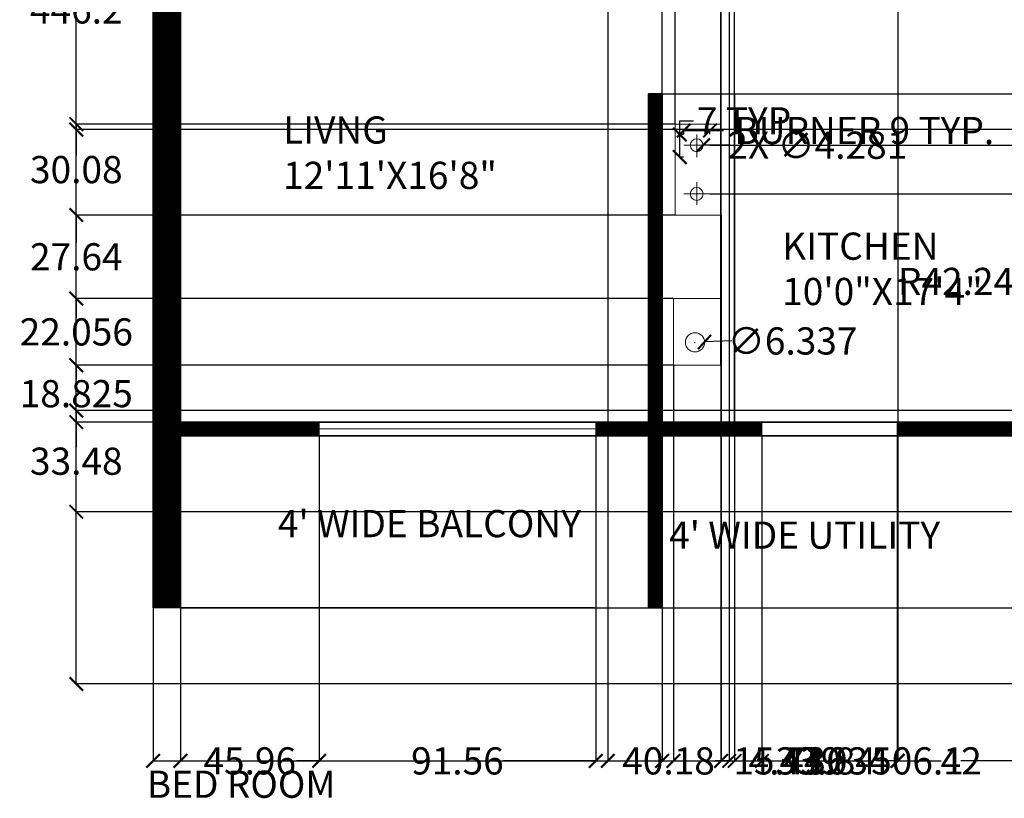
# Model space of a CAD drawing. Units: inches. Extents: x -43 to 552, y 22 to 537.
# Tile 1 of 4: x -43 to 283, y 22 to 280. Entities that reach past the tile are written whole.
import ezdxf

# ---------------------------------------------------------------- set-up
doc = ezdxf.new("R2010")
doc.units = ezdxf.units.IN
doc.header["$MEASUREMENT"] = 0
for name, color, linetype, lineweight in [('A-ANNO-DIMS', 2, 'Continuous', 18), ('A-AREA-IDEN', 7, 'Continuous', 18), ('A-EQPM', 8, 'Continuous', 18), ('A-FLOR', 7, 'Continuous', 25), ('A-FLOR-CASE', 8, 'Continuous', 25), ('A-FLOR-FIXT', 9, 'Continuous', 18), ('A-GLAZ', 4, 'Continuous', 18), ('A-WALL', 7, 'Continuous', 35), ('A-WALL-PATT', 252, 'Continuous', 13)]:
    doc.layers.add(name, color=color, linetype=linetype, lineweight=lineweight)
doc.styles.get("Standard").update_dxf_attribs({"font": 'arial.ttf'})
doc.dimstyles.get("Standard").update_dxf_attribs({"dimtxt": 9, "dimasz": 4.5, "dimexe": 0.18, "dimexo": 0.0625, "dimgap": 0.09, "dimtad": 0, "dimtih": 1, "dimtoh": 1, "dimdec": 1, "dimzin": 0, "dimdsep": 46, "dimlunit": 4, "dimtxsty": 'Standard', "dimblk": 'ARCHTICK', "dimcen": 0.09, "dimadec": 0, "dimazin": 0, "dimtfac": 1, "dimtdec": 1, "dimtofl": 0, "dimtmove": 0, "dimatfit": 3, "dimfxl": 1, "dimtolj": 1, "dimtzin": 0, "dimarcsym": 0})

# ---------------------------------------------------------------- blocks, each defined once
blk = doc.blocks.new('COOKTOP-BURNER')
for p, q in [((0, 0), (0, 3.57)), ((0, 3.57), (0, 0)), ((0, 0), (-4.28, 0)), ((0, 0), (4.4, 0)), ((0, 0), (0, -3.9))]:
    blk.add_line(p, q)
blk.add_circle((0, 0), 2.14)
blk = doc.blocks.new('_ArchTick')
at = {"color": 0, "linetype": 'ByBlock', "const_width": 0.15}
blk.add_lwpolyline([(-0.5, -0.5), (0.5, 0.5)], dxfattribs=at)
blk = doc.blocks.new('*D6')
at = {"layer": 'A-ANNO-DIMS', "color": 0, "lineweight": -2, "transparency": 16777216}
for p, q in [((177.13, 241.7), (177.13, 243.12)), ((177.13, 242.94), (185.81, 242.94)), ((185.81, 241.7), (185.81, 243.12)), ((185.81, 242.94), (190.31, 242.94))]:
    blk.add_line(p, q, dxfattribs=at)
at = {"layer": 'Defpoints', "color": 0, "transparency": 16777216}
for p in [(177.13, 241.64), (185.81, 242.94), (185.81, 241.64)]:
    blk.add_point(p, dxfattribs=at)
at = {"layer": 'A-ANNO-DIMS', "color": 0, "lineweight": -2, "transparency": 16777216, "xscale": 4.5, "yscale": 4.5, "zscale": 4.5, "rotation": 180}
blk.add_blockref('_ArchTick', (177.13, 242.94), dxfattribs=at)
at = {"layer": 'A-ANNO-DIMS', "color": 0, "lineweight": -2, "transparency": 16777216, "xscale": 4.5, "yscale": 4.5, "zscale": 4.5}
blk.add_blockref('_ArchTick', (185.81, 242.94), dxfattribs=at)
at = {"layer": 'A-ANNO-DIMS', "color": 0, "transparency": 16777216, "insert": (236.9, 242.94), "char_height": 9, "attachment_point": 5}
blk.add_mtext('\\A1;BURNER 9 TYP.', dxfattribs=at)
blk = doc.blocks.new('*D7')
at = {"layer": 'A-ANNO-DIMS', "color": 0, "lineweight": -2, "transparency": 16777216}
for p, q in [((175.83, 241.64), (175.83, 246.14)), ((175.83, 246.14), (180.33, 246.14)), ((177.07, 241.64), (175.65, 241.64)), ((175.83, 234.16), (175.83, 241.64)), ((177.07, 234.16), (175.65, 234.16))]:
    blk.add_line(p, q, dxfattribs=at)
at = {"layer": 'Defpoints', "color": 0, "transparency": 16777216}
for p in [(175.83, 241.64), (177.13, 241.64), (177.13, 234.16)]:
    blk.add_point(p, dxfattribs=at)
at = {"layer": 'A-ANNO-DIMS', "color": 0, "lineweight": -2, "transparency": 16777216, "xscale": 4.5, "yscale": 4.5, "zscale": 4.5}
for p, rotation in [((175.83, 241.64), 90), ((175.83, 234.16), 270)]:
    blk.add_blockref('_ArchTick', p, dxfattribs=dict(at, rotation=rotation))
at = {"layer": 'A-ANNO-DIMS', "color": 0, "transparency": 16777216, "insert": (198.79, 246.14), "char_height": 9, "attachment_point": 5}
blk.add_mtext('\\A1;7 TYP.', dxfattribs=at)
blk = doc.blocks.new('*D8')
at = {"layer": 'A-ANNO-DIMS', "color": 0, "lineweight": -2, "transparency": 16777216}
for p, q in [((507.56, 238.71), (507.56, 34.14)), ((1.46, 84.88), (1.46, 34.14)), ((1.46, 34.32), (240.11, 34.32)), ((507.56, 34.32), (268.92, 34.32))]:
    blk.add_line(p, q, dxfattribs=at)
at = {"layer": 'Defpoints', "color": 0, "transparency": 16777216}
for p in [(507.56, 238.77), (1.46, 84.95), (507.56, 34.32)]:
    blk.add_point(p, dxfattribs=at)
at = {"layer": 'A-ANNO-DIMS', "color": 0, "lineweight": -2, "transparency": 16777216, "xscale": 4.5, "yscale": 4.5, "zscale": 4.5, "rotation": 180}
blk.add_blockref('_ArchTick', (1.46, 34.32), dxfattribs=at)
at = {"layer": 'A-ANNO-DIMS', "color": 0, "lineweight": -2, "transparency": 16777216, "xscale": 4.5, "yscale": 4.5, "zscale": 4.5}
blk.add_blockref('_ArchTick', (507.56, 34.32), dxfattribs=at)
at = {"layer": 'A-ANNO-DIMS', "color": 0, "transparency": 16777216, "insert": (254.51, 34.32), "char_height": 9, "attachment_point": 5}
blk.add_mtext('\\A1;506.1', dxfattribs=at)
blk = doc.blocks.new('*D9')
at = {"layer": 'A-ANNO-DIMS', "color": 0, "lineweight": -2, "transparency": 16777216}
for p, q in [((82.45, 505.95), (-24.17, 505.95)), ((-23.99, 505.95), (-23.99, 287.55)), ((-23.99, 59.77), (-23.99, 278.18)), ((289.95, 59.77), (-24.17, 59.77))]:
    blk.add_line(p, q, dxfattribs=at)
at = {"layer": 'Defpoints', "color": 0, "transparency": 16777216}
for p in [(-23.99, 505.95), (82.51, 505.95), (290.01, 59.77)]:
    blk.add_point(p, dxfattribs=at)
at = {"layer": 'A-ANNO-DIMS', "color": 0, "lineweight": -2, "transparency": 16777216, "xscale": 4.5, "yscale": 4.5, "zscale": 4.5}
for p, rotation in [((-23.99, 505.95), 90), ((-23.99, 59.77), 270)]:
    blk.add_blockref('_ArchTick', p, dxfattribs=dict(at, rotation=rotation))
at = {"layer": 'A-ANNO-DIMS', "color": 0, "transparency": 16777216, "insert": (-23.99, 282.86), "char_height": 9, "attachment_point": 5}
blk.add_mtext('\\A1;446.2', dxfattribs=at)
blk = doc.blocks.new('*D22')
at = {"layer": 'A-ANNO-DIMS', "color": 0, "lineweight": -2, "transparency": 16777216}
for p, q in [((10.46, 141.88), (10.46, 34.14)), ((56.42, 141.88), (56.42, 34.14)), ((10.46, 34.32), (17.99, 34.32)), ((56.42, 34.32), (48.9, 34.32))]:
    blk.add_line(p, q, dxfattribs=at)
at = {"layer": 'Defpoints', "color": 0, "transparency": 16777216}
for p in [(10.46, 141.95), (56.42, 141.95), (56.42, 34.32)]:
    blk.add_point(p, dxfattribs=at)
at = {"layer": 'A-ANNO-DIMS', "color": 0, "lineweight": -2, "transparency": 16777216, "xscale": 4.5, "yscale": 4.5, "zscale": 4.5, "rotation": 180}
blk.add_blockref('_ArchTick', (10.46, 34.32), dxfattribs=at)
at = {"layer": 'A-ANNO-DIMS', "color": 0, "lineweight": -2, "transparency": 16777216, "xscale": 4.5, "yscale": 4.5, "zscale": 4.5}
blk.add_blockref('_ArchTick', (56.42, 34.32), dxfattribs=at)
at = {"layer": 'A-ANNO-DIMS', "color": 0, "transparency": 16777216, "insert": (33.44, 34.32), "char_height": 9, "attachment_point": 5}
blk.add_mtext('\\A1;45.96', dxfattribs=at)
blk = doc.blocks.new('*D23')
at = {"layer": 'A-ANNO-DIMS', "color": 0, "lineweight": -2, "transparency": 16777216}
for p, q in [((56.42, 141.88), (56.42, 34.14)), ((147.98, 141.88), (147.98, 34.14)), ((56.42, 34.32), (86.93, 34.32)), ((147.98, 34.32), (117.47, 34.32))]:
    blk.add_line(p, q, dxfattribs=at)
at = {"layer": 'Defpoints', "color": 0, "transparency": 16777216}
for p in [(56.42, 141.95), (147.98, 141.95), (147.98, 34.32)]:
    blk.add_point(p, dxfattribs=at)
at = {"layer": 'A-ANNO-DIMS', "color": 0, "lineweight": -2, "transparency": 16777216, "xscale": 4.5, "yscale": 4.5, "zscale": 4.5, "rotation": 180}
blk.add_blockref('_ArchTick', (56.42, 34.32), dxfattribs=at)
at = {"layer": 'A-ANNO-DIMS', "color": 0, "lineweight": -2, "transparency": 16777216, "xscale": 4.5, "yscale": 4.5, "zscale": 4.5}
blk.add_blockref('_ArchTick', (147.98, 34.32), dxfattribs=at)
at = {"layer": 'A-ANNO-DIMS', "color": 0, "transparency": 16777216, "insert": (102.2, 34.32), "char_height": 9, "attachment_point": 5}
blk.add_mtext('\\A1;91.56', dxfattribs=at)
blk = doc.blocks.new('*D26')
at = {"layer": 'A-ANNO-DIMS', "color": 0, "lineweight": -2, "transparency": 16777216}
for p, q in [((203, 141.88), (203, 34.14)), ((247.84, 141.88), (247.84, 34.14)), ((203, 34.32), (209.98, 34.32)), ((247.84, 34.32), (240.86, 34.32))]:
    blk.add_line(p, q, dxfattribs=at)
at = {"layer": 'Defpoints', "color": 0, "transparency": 16777216}
for p in [(203, 141.95), (247.84, 141.95), (247.84, 34.32)]:
    blk.add_point(p, dxfattribs=at)
at = {"layer": 'A-ANNO-DIMS', "color": 0, "lineweight": -2, "transparency": 16777216, "xscale": 4.5, "yscale": 4.5, "zscale": 4.5, "rotation": 180}
blk.add_blockref('_ArchTick', (203, 34.32), dxfattribs=at)
at = {"layer": 'A-ANNO-DIMS', "color": 0, "lineweight": -2, "transparency": 16777216, "xscale": 4.5, "yscale": 4.5, "zscale": 4.5}
blk.add_blockref('_ArchTick', (247.84, 34.32), dxfattribs=at)
at = {"layer": 'A-ANNO-DIMS', "color": 0, "transparency": 16777216, "insert": (225.42, 34.32), "char_height": 9, "attachment_point": 5}
blk.add_mtext('\\A1;44.84', dxfattribs=at)
blk = doc.blocks.new('*D27')
at = {"layer": 'A-ANNO-DIMS', "color": 0, "lineweight": -2, "transparency": 16777216}
for p, q in [((169.96, 141.88), (169.96, 34.14)), ((203, 141.88), (203, 34.14)), ((169.96, 34.32), (203, 34.32)), ((203, 34.32), (207.5, 34.32))]:
    blk.add_line(p, q, dxfattribs=at)
at = {"layer": 'Defpoints', "color": 0, "transparency": 16777216}
for p in [(169.96, 141.95), (203, 141.95), (203, 34.32)]:
    blk.add_point(p, dxfattribs=at)
at = {"layer": 'A-ANNO-DIMS', "color": 0, "lineweight": -2, "transparency": 16777216, "xscale": 4.5, "yscale": 4.5, "zscale": 4.5, "rotation": 180}
blk.add_blockref('_ArchTick', (169.96, 34.32), dxfattribs=at)
at = {"layer": 'A-ANNO-DIMS', "color": 0, "lineweight": -2, "transparency": 16777216, "xscale": 4.5, "yscale": 4.5, "zscale": 4.5}
blk.add_blockref('_ArchTick', (203, 34.32), dxfattribs=at)
at = {"layer": 'A-ANNO-DIMS', "color": 0, "transparency": 16777216, "insert": (226.25, 34.32), "char_height": 9, "attachment_point": 5}
blk.add_mtext('\\A1;33.034', dxfattribs=at)
blk = doc.blocks.new('*D29')
at = {"layer": 'A-ANNO-DIMS', "color": 0, "lineweight": -2, "transparency": 16777216}
for p, q in [((364.95, 346.45), (-24.17, 346.45)), ((-23.99, 346.45), (-23.99, 299.55)), ((-23.99, 243.27), (-23.99, 290.17)), ((364.95, 243.27), (-24.17, 243.27))]:
    blk.add_line(p, q, dxfattribs=at)
at = {"layer": 'Defpoints', "color": 0, "transparency": 16777216}
for p in [(-23.99, 346.45), (365.01, 346.45), (365.01, 243.27)]:
    blk.add_point(p, dxfattribs=at)
at = {"layer": 'A-ANNO-DIMS', "color": 0, "lineweight": -2, "transparency": 16777216, "xscale": 4.5, "yscale": 4.5, "zscale": 4.5}
for p, rotation in [((-23.99, 346.45), 90), ((-23.99, 243.27), 270)]:
    blk.add_blockref('_ArchTick', p, dxfattribs=dict(at, rotation=rotation))
at = {"layer": 'A-ANNO-DIMS', "color": 0, "transparency": 16777216, "insert": (-23.99, 294.86), "char_height": 9, "attachment_point": 5}
blk.add_mtext('\\A1;103.17', dxfattribs=at)
blk = doc.blocks.new('*D35')
at = {"layer": 'A-ANNO-DIMS', "color": 0, "lineweight": -2, "transparency": 16777216}
for p, q in [((10.53, 141.95), (533.19, 141.95)), ((533.01, 141.95), (533.01, 118.11)), ((533.01, 84.95), (533.01, 108.78)), ((10.53, 84.95), (533.19, 84.95))]:
    blk.add_line(p, q, dxfattribs=at)
at = {"layer": 'Defpoints', "color": 0, "transparency": 16777216}
for p in [(10.46, 141.95), (533.01, 141.95), (10.46, 84.95)]:
    blk.add_point(p, dxfattribs=at)
at = {"layer": 'A-ANNO-DIMS', "color": 0, "lineweight": -2, "transparency": 16777216, "xscale": 4.5, "yscale": 4.5, "zscale": 4.5}
for p, rotation in [((533.01, 141.95), 90), ((533.01, 84.95), 270)]:
    blk.add_blockref('_ArchTick', p, dxfattribs=dict(at, rotation=rotation))
at = {"layer": 'A-ANNO-DIMS', "color": 0, "transparency": 16777216, "insert": (533.01, 113.45), "char_height": 9, "attachment_point": 5}
blk.add_mtext('\\A1;57', dxfattribs=at)
blk = doc.blocks.new('*D37')
at = {"layer": 'A-ANNO-DIMS', "color": 0, "lineweight": -2, "transparency": 16777216}
for p, q in [((248.01, 346.38), (248.01, 34.14)), ((290.01, 346.38), (290.01, 34.14)), ((248.01, 34.32), (262.34, 34.32)), ((290.01, 34.32), (275.68, 34.32))]:
    blk.add_line(p, q, dxfattribs=at)
at = {"layer": 'Defpoints', "color": 0, "transparency": 16777216}
for p in [(248.01, 346.45), (290.01, 346.45), (290.01, 34.32)]:
    blk.add_point(p, dxfattribs=at)
at = {"layer": 'A-ANNO-DIMS', "color": 0, "lineweight": -2, "transparency": 16777216, "xscale": 4.5, "yscale": 4.5, "zscale": 4.5, "rotation": 180}
blk.add_blockref('_ArchTick', (248.01, 34.32), dxfattribs=at)
at = {"layer": 'A-ANNO-DIMS', "color": 0, "lineweight": -2, "transparency": 16777216, "xscale": 4.5, "yscale": 4.5, "zscale": 4.5}
blk.add_blockref('_ArchTick', (290.01, 34.32), dxfattribs=at)
at = {"layer": 'A-ANNO-DIMS', "color": 0, "transparency": 16777216, "insert": (269.01, 34.32), "char_height": 9, "attachment_point": 5}
blk.add_mtext('\\A1;42', dxfattribs=at)
blk = doc.blocks.new('*D39')
at = {"layer": 'A-ANNO-DIMS', "color": 0, "lineweight": -2, "transparency": 16777216}
for p, q in [((152.01, 496.88), (152.01, 34.14)), ((192.19, 486.68), (192.19, 34.14)), ((152.01, 34.32), (156.63, 34.32)), ((192.19, 34.32), (187.56, 34.32))]:
    blk.add_line(p, q, dxfattribs=at)
at = {"layer": 'Defpoints', "color": 0, "transparency": 16777216}
for p in [(152.01, 496.95), (192.19, 486.74), (192.19, 34.32)]:
    blk.add_point(p, dxfattribs=at)
at = {"layer": 'A-ANNO-DIMS', "color": 0, "lineweight": -2, "transparency": 16777216, "xscale": 4.5, "yscale": 4.5, "zscale": 4.5, "rotation": 180}
blk.add_blockref('_ArchTick', (152.01, 34.32), dxfattribs=at)
at = {"layer": 'A-ANNO-DIMS', "color": 0, "lineweight": -2, "transparency": 16777216, "xscale": 4.5, "yscale": 4.5, "zscale": 4.5}
blk.add_blockref('_ArchTick', (192.19, 34.32), dxfattribs=at)
at = {"layer": 'A-ANNO-DIMS', "color": 0, "transparency": 16777216, "insert": (172.1, 34.32), "char_height": 9, "attachment_point": 5}
blk.add_mtext('\\A1;40.18', dxfattribs=at)
blk = doc.blocks.new('*D43')
at = {"layer": 'A-ANNO-DIMS', "color": 0, "lineweight": -2, "transparency": 16777216}
for p, q in [((449.17, 150.25), (-24.17, 150.25)), ((-23.99, 150.25), (-23.99, 138.2)), ((-23.99, 116.77), (-23.99, 128.83)), ((468.45, 116.77), (-24.17, 116.77))]:
    blk.add_line(p, q, dxfattribs=at)
at = {"layer": 'Defpoints', "color": 0, "transparency": 16777216}
for p in [(-23.99, 150.25), (449.23, 150.25), (468.51, 116.77)]:
    blk.add_point(p, dxfattribs=at)
at = {"layer": 'A-ANNO-DIMS', "color": 0, "lineweight": -2, "transparency": 16777216, "xscale": 4.5, "yscale": 4.5, "zscale": 4.5}
for p, rotation in [((-23.99, 150.25), 90), ((-23.99, 116.77), 270)]:
    blk.add_blockref('_ArchTick', p, dxfattribs=dict(at, rotation=rotation))
at = {"layer": 'A-ANNO-DIMS', "color": 0, "transparency": 16777216, "insert": (-23.99, 133.51), "char_height": 9, "attachment_point": 5}
blk.add_mtext('\\A1;33.48', dxfattribs=at)
blk = doc.blocks.new('*D44')
at = {"layer": 'A-ANNO-DIMS', "color": 0, "lineweight": -2, "transparency": 16777216}
for p, q in [((169.96, 255.18), (169.96, 531.58)), ((169.96, 531.4), (175.37, 531.4)), ((193.96, 531.4), (188.56, 531.4)), ((193.96, 255.18), (193.96, 531.58))]:
    blk.add_line(p, q, dxfattribs=at)
at = {"layer": 'Defpoints', "color": 0, "transparency": 16777216}
for p in [(193.96, 531.4), (169.96, 255.12), (193.96, 255.12)]:
    blk.add_point(p, dxfattribs=at)
at = {"layer": 'A-ANNO-DIMS', "color": 0, "lineweight": -2, "transparency": 16777216, "xscale": 4.5, "yscale": 4.5, "zscale": 4.5, "rotation": 180}
blk.add_blockref('_ArchTick', (169.96, 531.4), dxfattribs=at)
at = {"layer": 'A-ANNO-DIMS', "color": 0, "lineweight": -2, "transparency": 16777216, "xscale": 4.5, "yscale": 4.5, "zscale": 4.5}
blk.add_blockref('_ArchTick', (193.96, 531.4), dxfattribs=at)
at = {"layer": 'A-ANNO-DIMS', "color": 0, "transparency": 16777216, "insert": (181.96, 531.4), "char_height": 9, "attachment_point": 5}
blk.add_mtext('\\A1;24', dxfattribs=at)
blk = doc.blocks.new('*D45')
at = {"layer": 'A-ANNO-DIMS', "color": 0, "lineweight": -2, "transparency": 16777216}
for p, q in [((194.03, 255.12), (533.19, 255.12)), ((533.01, 255.12), (533.01, 205.47)), ((533.01, 146.45), (533.01, 196.1)), ((194.03, 146.45), (533.19, 146.45))]:
    blk.add_line(p, q, dxfattribs=at)
at = {"layer": 'Defpoints', "color": 0, "transparency": 16777216}
for p in [(193.96, 255.12), (533.01, 255.12), (193.96, 146.45)]:
    blk.add_point(p, dxfattribs=at)
at = {"layer": 'A-ANNO-DIMS', "color": 0, "lineweight": -2, "transparency": 16777216, "xscale": 4.5, "yscale": 4.5, "zscale": 4.5}
for p, rotation in [((533.01, 255.12), 90), ((533.01, 146.45), 270)]:
    blk.add_blockref('_ArchTick', p, dxfattribs=dict(at, rotation=rotation))
at = {"layer": 'A-ANNO-DIMS', "color": 0, "transparency": 16777216, "insert": (533.01, 200.78), "char_height": 9, "attachment_point": 5}
blk.add_mtext('\\A1;108.67', dxfattribs=at)
blk = doc.blocks.new('*D46')
at = {"layer": 'A-ANNO-DIMS', "color": 0, "lineweight": -2, "transparency": 16777216}
for p, q in [((173.71, 165.21), (173.71, 34.14)), ((189.45, 165.21), (189.45, 34.14)), ((173.71, 34.32), (189.45, 34.32)), ((189.45, 34.32), (193.95, 34.32))]:
    blk.add_line(p, q, dxfattribs=at)
at = {"layer": 'Defpoints', "color": 0, "transparency": 16777216}
for p in [(173.71, 165.27), (189.45, 165.27), (189.45, 34.32)]:
    blk.add_point(p, dxfattribs=at)
at = {"layer": 'A-ANNO-DIMS', "color": 0, "lineweight": -2, "transparency": 16777216, "xscale": 4.5, "yscale": 4.5, "zscale": 4.5, "rotation": 180}
blk.add_blockref('_ArchTick', (173.71, 34.32), dxfattribs=at)
at = {"layer": 'A-ANNO-DIMS', "color": 0, "lineweight": -2, "transparency": 16777216, "xscale": 4.5, "yscale": 4.5, "zscale": 4.5}
blk.add_blockref('_ArchTick', (189.45, 34.32), dxfattribs=at)
at = {"layer": 'A-ANNO-DIMS', "color": 0, "transparency": 16777216, "insert": (212.29, 34.32), "char_height": 9, "attachment_point": 5}
blk.add_mtext('\\A1;15.736', dxfattribs=at)
blk = doc.blocks.new('*D47')
at = {"layer": 'A-ANNO-DIMS', "color": 0, "lineweight": -2, "transparency": 16777216}
for p, q in [((173.65, 187.33), (-24.17, 187.33)), ((-23.99, 187.33), (-23.99, 180.99)), ((-23.99, 165.27), (-23.99, 171.62)), ((173.65, 165.27), (-24.17, 165.27))]:
    blk.add_line(p, q, dxfattribs=at)
at = {"layer": 'Defpoints', "color": 0, "transparency": 16777216}
for p in [(-23.99, 187.33), (173.71, 187.33), (173.71, 165.27)]:
    blk.add_point(p, dxfattribs=at)
at = {"layer": 'A-ANNO-DIMS', "color": 0, "lineweight": -2, "transparency": 16777216, "xscale": 4.5, "yscale": 4.5, "zscale": 4.5}
for p, rotation in [((-23.99, 187.33), 90), ((-23.99, 165.27), 270)]:
    blk.add_blockref('_ArchTick', p, dxfattribs=dict(at, rotation=rotation))
at = {"layer": 'A-ANNO-DIMS', "color": 0, "transparency": 16777216, "insert": (-23.99, 176.3), "char_height": 9, "attachment_point": 5}
blk.add_mtext('\\A1;22.056', dxfattribs=at)
blk = doc.blocks.new('*D48')
at = {"layer": 'A-ANNO-DIMS', "color": 0, "lineweight": -2, "transparency": 16777216}
for p, q in [((174.25, 245.05), (-24.17, 245.05)), ((-23.99, 245.05), (-23.99, 234.7)), ((-23.99, 214.97), (-23.99, 225.32)), ((174.25, 214.97), (-24.17, 214.97))]:
    blk.add_line(p, q, dxfattribs=at)
at = {"layer": 'Defpoints', "color": 0, "transparency": 16777216}
for p in [(-23.99, 245.05), (174.31, 245.05), (174.31, 214.97)]:
    blk.add_point(p, dxfattribs=at)
at = {"layer": 'A-ANNO-DIMS', "color": 0, "lineweight": -2, "transparency": 16777216, "xscale": 4.5, "yscale": 4.5, "zscale": 4.5}
for p, rotation in [((-23.99, 245.05), 90), ((-23.99, 214.97), 270)]:
    blk.add_blockref('_ArchTick', p, dxfattribs=dict(at, rotation=rotation))
at = {"layer": 'A-ANNO-DIMS', "color": 0, "transparency": 16777216, "insert": (-23.99, 230.01), "char_height": 9, "attachment_point": 5}
blk.add_mtext('\\A1;30.08', dxfattribs=at)
blk = doc.blocks.new('*D49')
at = {"layer": 'A-ANNO-DIMS', "color": 0, "lineweight": -2, "transparency": 16777216}
for p, q in [((174.31, 245.11), (174.31, 531.58)), ((174.31, 531.4), (189.53, 531.4)), ((189.53, 245.11), (189.53, 531.58)), ((189.53, 531.4), (194.03, 531.4))]:
    blk.add_line(p, q, dxfattribs=at)
at = {"layer": 'Defpoints', "color": 0, "transparency": 16777216}
for p in [(189.53, 531.4), (174.31, 245.05), (189.53, 245.05)]:
    blk.add_point(p, dxfattribs=at)
at = {"layer": 'A-ANNO-DIMS', "color": 0, "lineweight": -2, "transparency": 16777216, "xscale": 4.5, "yscale": 4.5, "zscale": 4.5, "rotation": 180}
blk.add_blockref('_ArchTick', (174.31, 531.4), dxfattribs=at)
at = {"layer": 'A-ANNO-DIMS', "color": 0, "lineweight": -2, "transparency": 16777216, "xscale": 4.5, "yscale": 4.5, "zscale": 4.5}
blk.add_blockref('_ArchTick', (189.53, 531.4), dxfattribs=at)
at = {"layer": 'A-ANNO-DIMS', "color": 0, "transparency": 16777216, "insert": (212.37, 531.4), "char_height": 9, "attachment_point": 5}
blk.add_mtext('\\A1;15.216', dxfattribs=at)
blk = doc.blocks.new('*D50')
at = {"layer": 'A-ANNO-DIMS', "color": 0, "lineweight": -2, "transparency": 16777216}
for p, q in [((173.65, 165.27), (-24.17, 165.27)), ((-23.99, 165.27), (-23.99, 160.55)), ((-23.99, 146.45), (-23.99, 151.17)), ((169.9, 146.45), (-24.17, 146.45))]:
    blk.add_line(p, q, dxfattribs=at)
at = {"layer": 'Defpoints', "color": 0, "transparency": 16777216}
for p in [(-23.99, 165.27), (173.71, 165.27), (169.96, 146.45)]:
    blk.add_point(p, dxfattribs=at)
at = {"layer": 'A-ANNO-DIMS', "color": 0, "lineweight": -2, "transparency": 16777216, "xscale": 4.5, "yscale": 4.5, "zscale": 4.5}
for p, rotation in [((-23.99, 165.27), 90), ((-23.99, 146.45), 270)]:
    blk.add_blockref('_ArchTick', p, dxfattribs=dict(at, rotation=rotation))
at = {"layer": 'A-ANNO-DIMS', "color": 0, "transparency": 16777216, "insert": (-23.99, 155.86), "char_height": 9, "attachment_point": 5}
blk.add_mtext('\\A1;18.825', dxfattribs=at)
blk = doc.blocks.new('*D51')
at = {"layer": 'A-ANNO-DIMS', "color": 0, "lineweight": -2, "transparency": 16777216}
for p, q in [((174.25, 214.97), (-24.17, 214.97)), ((-23.99, 214.97), (-23.99, 205.83)), ((-23.99, 187.33), (-23.99, 196.46)), ((173.65, 187.33), (-24.17, 187.33))]:
    blk.add_line(p, q, dxfattribs=at)
at = {"layer": 'Defpoints', "color": 0, "transparency": 16777216}
for p in [(-23.99, 214.97), (174.31, 214.97), (173.71, 187.33)]:
    blk.add_point(p, dxfattribs=at)
at = {"layer": 'A-ANNO-DIMS', "color": 0, "lineweight": -2, "transparency": 16777216, "xscale": 4.5, "yscale": 4.5, "zscale": 4.5}
for p, rotation in [((-23.99, 214.97), 90), ((-23.99, 187.33), 270)]:
    blk.add_blockref('_ArchTick', p, dxfattribs=dict(at, rotation=rotation))
at = {"layer": 'A-ANNO-DIMS', "color": 0, "transparency": 16777216, "insert": (-23.99, 201.15), "char_height": 9, "attachment_point": 5}
blk.add_mtext('\\A1;27.64', dxfattribs=at)
blk = doc.blocks.new('*D52')
at = {"layer": 'A-ANNO-DIMS', "color": 0, "lineweight": -2, "transparency": 16777216}
for p, q in [((193.96, 255.05), (193.96, 34.14)), ((189.53, 214.91), (189.53, 34.14)), ((189.53, 34.32), (193.96, 34.32)), ((193.96, 34.32), (198.46, 34.32))]:
    blk.add_line(p, q, dxfattribs=at)
at = {"layer": 'Defpoints', "color": 0, "transparency": 16777216}
for p in [(193.96, 255.12), (189.53, 214.97), (193.96, 34.32)]:
    blk.add_point(p, dxfattribs=at)
at = {"layer": 'A-ANNO-DIMS', "color": 0, "lineweight": -2, "transparency": 16777216, "xscale": 4.5, "yscale": 4.5, "zscale": 4.5, "rotation": 180}
blk.add_blockref('_ArchTick', (189.53, 34.32), dxfattribs=at)
at = {"layer": 'A-ANNO-DIMS', "color": 0, "lineweight": -2, "transparency": 16777216, "xscale": 4.5, "yscale": 4.5, "zscale": 4.5}
blk.add_blockref('_ArchTick', (193.96, 34.32), dxfattribs=at)
at = {"layer": 'A-ANNO-DIMS', "color": 0, "transparency": 16777216, "insert": (213.93, 34.32), "char_height": 9, "attachment_point": 5}
blk.add_mtext('\\A1;4.439', dxfattribs=at)
blk = doc.blocks.new('*D53')
at = {"layer": 'A-ANNO-DIMS', "color": 0, "lineweight": -2, "transparency": 16777216}
for p, q in [((189.45, 165.34), (189.45, 531.58)), ((189.45, 531.4), (193.96, 531.4)), ((193.96, 146.51), (193.96, 531.58)), ((193.96, 531.4), (198.46, 531.4))]:
    blk.add_line(p, q, dxfattribs=at)
at = {"layer": 'Defpoints', "color": 0, "transparency": 16777216}
for p in [(193.96, 531.4), (189.45, 165.27), (193.96, 146.45)]:
    blk.add_point(p, dxfattribs=at)
at = {"layer": 'A-ANNO-DIMS', "color": 0, "lineweight": -2, "transparency": 16777216, "xscale": 4.5, "yscale": 4.5, "zscale": 4.5, "rotation": 180}
blk.add_blockref('_ArchTick', (189.45, 531.4), dxfattribs=at)
at = {"layer": 'A-ANNO-DIMS', "color": 0, "lineweight": -2, "transparency": 16777216, "xscale": 4.5, "yscale": 4.5, "zscale": 4.5}
blk.add_blockref('_ArchTick', (193.96, 531.4), dxfattribs=at)
at = {"layer": 'A-ANNO-DIMS', "color": 0, "transparency": 16777216, "insert": (210.38, 531.4), "char_height": 9, "attachment_point": 5}
blk.add_mtext('\\A1;4.52', dxfattribs=at)
blk = doc.blocks.new('*D54')
at = {"layer": 'A-ANNO-DIMS', "color": 0, "lineweight": -2, "transparency": 16777216}
for p, q in [((185.87, 238.07), (533.19, 238.07)), ((533.01, 238.07), (533.01, 234.7)), ((533.01, 221.96), (533.01, 225.33)), ((185.87, 221.96), (533.19, 221.96))]:
    blk.add_line(p, q, dxfattribs=at)
at = {"layer": 'Defpoints', "color": 0, "transparency": 16777216}
for p in [(185.81, 238.07), (533.01, 238.07), (185.81, 221.96)]:
    blk.add_point(p, dxfattribs=at)
at = {"layer": 'A-ANNO-DIMS', "color": 0, "lineweight": -2, "transparency": 16777216, "xscale": 4.5, "yscale": 4.5, "zscale": 4.5}
for p, rotation in [((533.01, 238.07), 90), ((533.01, 221.96), 270)]:
    blk.add_blockref('_ArchTick', p, dxfattribs=dict(at, rotation=rotation))
at = {"layer": 'A-ANNO-DIMS', "color": 0, "transparency": 16777216, "insert": (533.01, 230.01), "char_height": 9, "attachment_point": 5}
blk.add_mtext('\\A1;16.11', dxfattribs=at)
blk = doc.blocks.new('*D57')
at = {"layer": 'A-ANNO-DIMS', "color": 0, "lineweight": -2, "transparency": 16777216}
for p, q in [((336.42, 243.27), (336.6, 243.27)), ((336.51, 243.18), (336.51, 243.36)), ((291.34, 193), (308.28, 211.86)), ((286.84, 193), (291.34, 193))]:
    blk.add_line(p, q, dxfattribs=at)
at = {"layer": 'Defpoints', "color": 0, "transparency": 16777216}
for p in [(336.51, 243.27), (308.28, 211.86)]:
    blk.add_point(p, dxfattribs=at)
at = {"layer": 'A-ANNO-DIMS', "color": 0, "lineweight": -2, "transparency": 16777216, "xscale": 4.5, "yscale": 4.5, "zscale": 4.5, "rotation": 48.05760462108148}
blk.add_blockref('_ArchTick', (308.28, 211.86), dxfattribs=at)
at = {"layer": 'A-ANNO-DIMS', "color": 0, "transparency": 16777216, "insert": (267.27, 193), "char_height": 9, "attachment_point": 5}
blk.add_mtext('\\A1;R42.24', dxfattribs=at)
blk = doc.blocks.new('*D59')
at = {"layer": 'A-ANNO-DIMS', "color": 0, "lineweight": -2, "transparency": 16777216}
for p, q in [((180.75, 172.84), (180.93, 172.84)), ((180.84, 172.75), (180.84, 172.93)), ((193, 173.3), (184.01, 172.96))]:
    blk.add_line(p, q, dxfattribs=at)
at = {"layer": 'Defpoints', "color": 0, "transparency": 16777216}
for p in [(184.01, 172.96), (177.68, 172.72)]:
    blk.add_point(p, dxfattribs=at)
at = {"layer": 'A-ANNO-DIMS', "color": 0, "lineweight": -2, "transparency": 16777216, "xscale": 4.5, "yscale": 4.5, "zscale": 4.5, "rotation": 182.1701531593034}
blk.add_blockref('_ArchTick', (184.01, 172.96), dxfattribs=at)
at = {"layer": 'A-ANNO-DIMS', "color": 0, "transparency": 16777216, "insert": (213.18, 173.3), "char_height": 9, "attachment_point": 5}
blk.add_mtext('\\A1;∅6.337', dxfattribs=at)
blk = doc.blocks.new('*D60')
at = {"layer": 'A-ANNO-DIMS', "color": 0, "lineweight": -2, "transparency": 16777216}
for p, q in [((181.32, 238.07), (181.5, 238.07)), ((181.41, 237.98), (181.41, 238.16)), ((192.55, 238.09), (183.55, 238.07))]:
    blk.add_line(p, q, dxfattribs=at)
at = {"layer": 'Defpoints', "color": 0, "transparency": 16777216}
for p in [(179.27, 238.06), (183.55, 238.07)]:
    blk.add_point(p, dxfattribs=at)
at = {"layer": 'A-ANNO-DIMS', "color": 0, "lineweight": -2, "transparency": 16777216, "xscale": 4.5, "yscale": 4.5, "zscale": 4.5, "rotation": 180.1229965869815}
blk.add_blockref('_ArchTick', (183.55, 238.07), dxfattribs=at)
at = {"layer": 'A-ANNO-DIMS', "color": 0, "transparency": 16777216, "insert": (221.36, 238.09), "char_height": 9, "attachment_point": 5}
blk.add_mtext('\\A1;2X ∅4.281', dxfattribs=at)

msp = doc.modelspace()

# ---------------------------------------------------------------- hatches: boundary and pattern name
at = {"layer": 'A-WALL-PATT'}
h = msp.add_hatch(dxfattribs=at)
h.set_pattern_fill('ANSI31', color=256)
h.set_pattern_definition([(45, (-523.11303, 0), (-0.088388348, 0.088388348), [])])
h.paths.add_polyline_path([(202.9985, 146.4471), (169.965, 146.4471), (169.965, 255.1157), (165.465, 255.1157), (165.465, 146.4471), (147.9805, 146.4471), (147.9805, 141.9471), (165.465, 141.9471), (165.465, 84.9471), (169.965, 84.9471), (169.965, 141.9471), (202.9985, 141.9471)])
h.paths.add_polyline_path([(294.5106, 146.4471), (294.5106, 238.775), (294.5106, 243.275), (294.5106, 255.1157), (290.0106, 255.1157), (290.0106, 146.4471), (247.8411, 146.4471), (247.8411, 141.9471), (290.0106, 141.9471), (290.0106, 93.9471), (290.0106, 59.775), (294.5106, 59.775), (294.5106, 77.3814), (294.5106, 93.9471), (294.5106, 107.775), (316.2676, 107.775), (316.2676, 116.775), (294.5106, 116.775)])
h.paths.add_polyline_path([(10.465, 346.4471), (82.5106, 346.4471), (91.5106, 346.4471), (91.5106, 358.2163), (82.5106, 358.2163), (82.5106, 350.9471), (1.465, 350.9471), (1.465, 84.9471), (10.465, 84.9471), (10.465, 141.9471), (56.4237, 141.9471), (56.4237, 146.4471), (10.465, 146.4471)])
h.paths.add_polyline_path([(91.5106, 496.9471), (107.5106, 496.9471), (107.5106, 505.9471), (82.5106, 505.9471), (82.5106, 400.4471), (147.5106, 400.4471), (147.5106, 346.4471), (248.0106, 346.4471), (248.0106, 350.9471), (152.0106, 350.9471), (152.0106, 496.9471), (197.0106, 496.9471), (197.0106, 505.9471), (131.5106, 505.9471), (131.5106, 496.9471), (147.5106, 496.9471), (147.5106, 404.9471), (91.5106, 404.9471)])
h.paths.add_polyline_path([(477.5106, 505.9471), (245.0106, 505.9471), (245.0106, 496.9471), (290.0106, 496.9471), (290.0106, 390.2693, -0.02565505), (294.5106, 390.2693), (294.5106, 496.9471), (468.5106, 496.9471), (468.5106, 460.1763), (477.5106, 460.1763)])

# ---------------------------------------------------------------- linework, layer by layer
at = {"layer": 'A-EQPM'}
for p, q in [((174.3101, 245.0503), (189.5259, 245.0503)), ((174.3101, 214.9706), (174.3101, 245.0503)), ((189.5259, 245.0503), (189.5259, 214.9706)), ((189.5259, 214.9706), (174.3101, 214.9706))]:
    msp.add_line(p, q, dxfattribs=at)
at = {"layer": 'A-FLOR'}
for q in [(1.465, 84.9471), (290.0106, 84.9471)]:
    msp.add_line((147.5106, 84.9471), q, dxfattribs=at)
at = {"layer": 'A-FLOR-CASE'}
for p, q in [((169.965, 255.1157), (193.965, 255.1157)), ((193.965, 255.1157), (193.965, 146.4471))]:
    msp.add_line(p, q, dxfattribs=at)
at = {"layer": 'A-FLOR-FIXT'}
msp.add_lwpolyline([(173.7137, 187.3286), (189.4495, 187.3286), (189.4495, 165.2726), (173.7137, 165.2726)], close=True, dxfattribs=at)
msp.add_circle((180.8445, 172.838), 3.1685, dxfattribs=at)
at = {"layer": 'A-GLAZ'}
for p, q in [((56.4237, 146.4471), (56.4237, 141.9471)), ((56.4237, 144.1971), (147.9805, 144.1971)), ((147.9805, 146.4471), (147.9805, 141.9471)), ((202.9985, 146.4471), (202.9985, 141.9471)), ((247.8411, 146.4471), (247.8411, 141.9471))]:
    msp.add_line(p, q, dxfattribs=at)
at = {"layer": 'A-WALL'}
for p, q in [((1.465, 350.9471), (1.465, 84.9471)), ((10.465, 346.4471), (10.465, 146.4471)), ((165.465, 255.1157), (165.465, 146.4471)), ((169.965, 255.1157), (165.465, 255.1157)), ((169.965, 255.1157), (169.965, 146.4471)), ((82.5106, 146.4471), (10.465, 146.4471)), ((82.5106, 146.4471), (165.465, 146.4471)), ((169.965, 146.4471), (290.0106, 146.4471)), ((82.5106, 141.9471), (10.465, 141.9471)), ((10.465, 141.9471), (10.465, 84.9471)), ((82.5106, 141.9471), (165.465, 141.9471)), ((165.465, 141.9471), (165.465, 84.9471)), ((169.965, 141.9471), (169.965, 84.9471)), ((169.965, 141.9471), (290.0106, 141.9471))]:
    msp.add_line(p, q, dxfattribs=at)

# ---------------------------------------------------------------- block references
at = {"layer": 'A-EQPM'}
msp.add_blockref('COOKTOP-BURNER', (181.4108, 238.0655), dxfattribs=at)
at = {"layer": 'A-EQPM', "extrusion": (0, 0, -1), "zscale": -1, "rotation": 180}
msp.add_blockref('COOKTOP-BURNER', (-181.4108, 221.9554), dxfattribs=at)

# ---------------------------------------------------------------- texts
at = {"layer": 'A-AREA-IDEN', "char_height": 9, "attachment_point": 1}
for s, insert in [('LIVNG\\P12\'11\'X16\'8"', (44.48, 247.6139)), ('KITCHEN\\P10\'0"X17\'4"', (209.721, 209.1705)), ("4' WIDE BALCONY", (42.7425, 117.3453)), ("4' WIDE UTILITY", (172.2793, 113.5372)), ('BED ROOM', (-0.6528, 31.0994))]:
    msp.add_mtext_dynamic_manual_height_columns(s, width=549.697564, gutter_width=1, heights=[0], dxfattribs=dict(at, insert=insert))

# ---------------------------------------------------------------- dimensions: what is measured, and where the dimension line sits
at = {"layer": 'A-ANNO-DIMS'}
for base, p1, p2, override, picture, middle in [((193.965, 531.3971), (169.965, 255.1157), (193.965, 255.1157), {"dimdec": 0, "dimlfac": 1, "dimrnd": 0, "dimzin": 0, "dimdsep": 46, "dimlunit": 2}, '*D44', (181.965, 531.3971)), ((189.5259, 531.3971), (174.3101, 245.0503), (189.5259, 245.0503), {"dimdec": 3, "dimlfac": 1, "dimrnd": 0, "dimzin": 0, "dimdsep": 46, "dimlunit": 2}, '*D49', (212.3707, 531.3971)), ((193.965, 531.3971), (189.4495, 165.2726), (193.965, 146.4471), {"dimdec": 2, "dimlfac": 1, "dimrnd": 0, "dimzin": 0, "dimdsep": 46, "dimlunit": 2}, '*D53', (210.379, 531.3971)), ((192.1876, 34.325), (152.0106, 496.9471), (192.1876, 486.7427), {"dimdec": 2, "dimlfac": 1, "dimrnd": 0, "dimzin": 0, "dimdsep": 46, "dimlunit": 2}, '*D39', (172.0991, 34.325)), ((290.0106, 34.325), (248.0106, 346.4471), (290.0106, 346.4471), {"dimdec": 0, "dimlfac": 1, "dimrnd": 0, "dimzin": 0, "dimdsep": 46, "dimlunit": 2}, '*D37', (269.0106, 34.325)), ((193.965, 34.325), (189.5259, 214.9706), (193.965, 255.1157), {"dimdec": 3, "dimlfac": 1, "dimrnd": 0, "dimzin": 0, "dimdsep": 46, "dimlunit": 2}, '*D52', (213.9305, 34.325)), ((507.5611, 34.325), (1.465, 84.9471), (507.5611, 238.775), {"dimdec": 1, "dimlfac": 1, "dimrnd": 0, "dimzin": 0, "dimdsep": 46, "dimlunit": 2}, '*D8', (254.513, 34.325)), ((189.4495, 34.325), (173.7137, 165.2726), (189.4495, 165.2726), {"dimdec": 3, "dimlfac": 1, "dimrnd": 0, "dimzin": 0, "dimdsep": 46, "dimlunit": 2}, '*D46', (212.2942, 34.325)), ((56.4237, 34.325), (10.465, 141.9471), (56.4237, 141.9471), {"dimdec": 2, "dimlfac": 1, "dimrnd": 0, "dimzin": 0, "dimdsep": 46, "dimlunit": 2}, '*D22', (33.4443, 34.325)), ((147.9805, 34.325), (56.4237, 141.9471), (147.9805, 141.9471), {"dimdec": 2, "dimlfac": 1, "dimrnd": 0, "dimzin": 0, "dimdsep": 46, "dimlunit": 2}, '*D23', (102.2021, 34.325)), ((202.99846, 34.32496), (169.96495, 141.94715), (202.99846, 141.94715), {"dimdec": 3, "dimlfac": 1, "dimrnd": 0, "dimzin": 0, "dimdsep": 46, "dimlunit": 2}, '*D27', (226.24842, 34.32496)), ((247.8411, 34.325), (202.9985, 141.9471), (247.8411, 141.9471), {"dimdec": 2, "dimlfac": 1, "dimrnd": 0, "dimzin": 0, "dimdsep": 46, "dimlunit": 2}, '*D26', (225.4198, 34.325))]:
    dim = msp.add_linear_dim(base=base, p1=p1, p2=p2, dimstyle='Standard', override=override, dxfattribs=at)
    dim.commit()
    dim.dimension.update_dxf_attribs({"geometry": picture, "text_midpoint": middle})
for base, p1, p2, override, picture, middle in [((-23.985, 505.9471), (290.0106, 59.775), (82.5106, 505.9471), {"dimdec": 1, "dimlfac": 1, "dimrnd": 0, "dimzin": 0, "dimdsep": 46, "dimlunit": 2}, '*D9', (-23.985, 282.8611)), ((-23.985, 346.4471), (365.0106, 243.275), (365.0106, 346.4471), {"dimdec": 2, "dimlfac": 1, "dimrnd": 0, "dimzin": 0, "dimdsep": 46, "dimlunit": 2}, '*D29', (-23.985, 294.8611)), ((533.0111, 255.1157), (193.965, 146.4471), (193.965, 255.1157), {"dimdec": 2, "dimlfac": 1, "dimrnd": 0, "dimzin": 0, "dimdsep": 46, "dimlunit": 2}, '*D45', (533.0111, 200.7814)), ((-23.985, 245.0503), (174.3101, 214.9706), (174.3101, 245.0503), {"dimdec": 2, "dimlfac": 1, "dimrnd": 0, "dimzin": 0, "dimdsep": 46, "dimlunit": 2}, '*D48', (-23.985, 230.0105)), ((533.0111, 238.0655), (185.8076, 221.9554), (185.8076, 238.0655), {"dimdec": 2, "dimlfac": 1, "dimrnd": 0, "dimzin": 0, "dimdsep": 46, "dimlunit": 2}, '*D54', (533.0111, 230.0105)), ((-23.985, 214.9706), (173.7137, 187.3286), (174.3101, 214.9706), {"dimdec": 2, "dimlfac": 1, "dimrnd": 0, "dimzin": 0, "dimdsep": 46, "dimlunit": 2}, '*D51', (-23.985, 201.1496)), ((-23.985, 187.3286), (173.7137, 165.2726), (173.7137, 187.3286), {"dimdec": 3, "dimlfac": 1, "dimrnd": 0, "dimzin": 0, "dimdsep": 46, "dimlunit": 2}, '*D47', (-23.985, 176.3006)), ((-23.98505, 165.27256), (169.96495, 146.44715), (173.71369, 165.27256), {"dimdec": 3, "dimlfac": 1, "dimrnd": 0, "dimzin": 0, "dimdsep": 46, "dimlunit": 2}, '*D50', (-23.98505, 155.85985)), ((-23.985, 150.2529), (468.5106, 116.775), (449.2346, 150.2529), {"dimdec": 2, "dimlfac": 1, "dimrnd": 0, "dimzin": 0, "dimdsep": 46, "dimlunit": 2}, '*D43', (-23.985, 133.5139)), ((533.0111, 141.9471), (10.465, 84.9471), (10.465, 141.9471), {"dimdec": 0, "dimlfac": 1, "dimrnd": 0, "dimzin": 0, "dimdsep": 46, "dimlunit": 2}, '*D35', (533.0111, 113.4471))]:
    dim = msp.add_linear_dim(base=base, p1=p1, p2=p2, angle=90, dimstyle='Standard', override=override, dxfattribs=at)
    dim.commit()
    dim.dimension.update_dxf_attribs({"geometry": picture, "text_midpoint": middle})
dim = msp.add_linear_dim(base=(185.8076, 242.9397), p1=(177.1301, 241.6381), p2=(185.8076, 241.6381), text='BURNER <> TYP.', dimstyle='Standard', override={"dimdec": 0, "dimlfac": 1, "dimrnd": 0, "dimzin": 0, "dimdsep": 46, "dimlunit": 2}, dxfattribs=at)
dim.commit()
dim.dimension.update_dxf_attribs({"geometry": '*D6', "text_midpoint": (236.8986, 242.9397)})
dim = msp.add_linear_dim(base=(175.8285, 241.6381), p1=(177.1301, 234.1635), p2=(177.1301, 241.6381), angle=90, text='<> TYP.', dimstyle='Standard', override={"dimdec": 0, "dimlfac": 1, "dimrnd": 0, "dimzin": 0, "dimdsep": 46, "dimlunit": 2}, dxfattribs=at)
dim.commit()
dim.dimension.update_dxf_attribs({"geometry": '*D7', "text_midpoint": (198.7899, 246.1381)})
dim = msp.add_diameter_dim_2p(p1=(179.2703, 238.0609), p2=(183.5513, 238.0701), text='2X <>', dimstyle='Standard', override={"dimdec": 3, "dimlfac": 1, "dimrnd": 0, "dimzin": 0, "dimdsep": 46, "dimlunit": 2}, dxfattribs=at)
dim.commit()
dim.dimension.update_dxf_attribs({"geometry": '*D60', "text_midpoint": (192.5513, 238.0894)})
dim = msp.add_radius_dim(center=(336.5106, 243.275), mpoint=(308.2779, 211.8558), dimstyle='Standard', override={"dimdec": 2, "dimlfac": 1, "dimrnd": 0, "dimzin": 0, "dimdsep": 46, "dimlunit": 2}, dxfattribs=at)
dim.commit()
dim.dimension.update_dxf_attribs({"geometry": '*D57', "text_midpoint": (267.2748, 193.0044), "dimtype": 164})
dim = msp.add_diameter_dim_2p(p1=(177.6783, 172.718), p2=(184.0107, 172.958), dimstyle='Standard', override={"dimdec": 3, "dimlfac": 1, "dimrnd": 0, "dimzin": 0, "dimdsep": 46, "dimlunit": 2}, dxfattribs=at)
dim.commit()
dim.dimension.update_dxf_attribs({"geometry": '*D59', "text_midpoint": (193.0042, 173.2988), "dimtype": 163})

doc.saveas('drawing.dxf')
